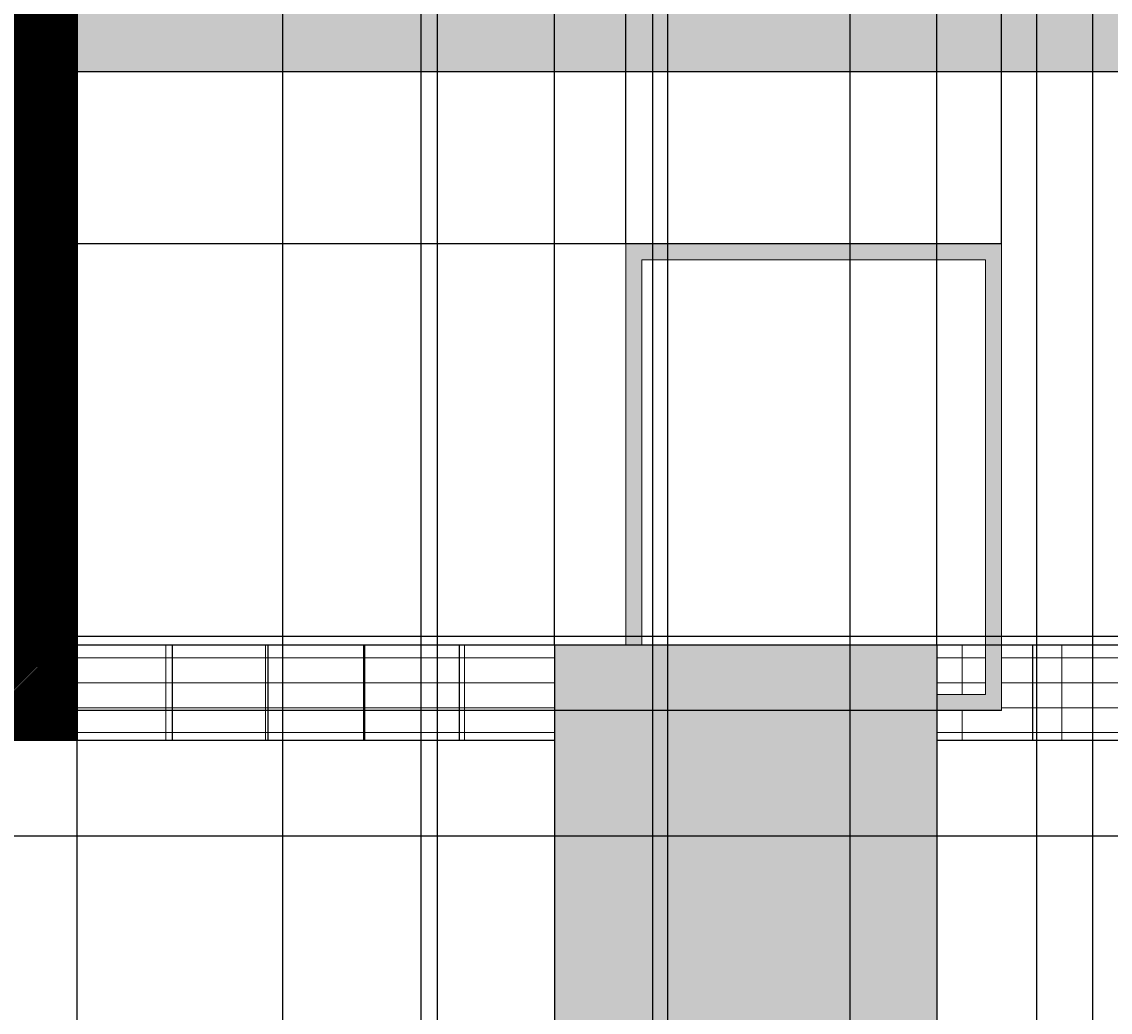
# Model space of a CAD drawing. Units: inches. Extents: x 484 to 1264, y 95 to 991.
# Tile 4 of 8: x 657 to 794, y 374 to 499. Entities that reach past the tile are written whole.
import ezdxf

# ---------------------------------------------------------------- set-up
doc = ezdxf.new("R2010")
doc.units = ezdxf.units.IN
doc.header["$MEASUREMENT"] = 0
for name, color, linetype, lineweight in [('A-ANNO-DIMS', 2, 'Continuous', 18), ('A-ELEV-TRIM', 7, 'Continuous', 18), ('A-GLAZ', 7, 'Continuous', 18), ('A-WALL', 7, 'Continuous', 35), ('L-FENC', 7, 'Continuous', 25), ('L-FENC-GRIL-PATT', 6, 'Continuous', 13)]:
    doc.layers.add(name, color=color, linetype=linetype, lineweight=lineweight)
for name, color, linetype, lineweight, true_color in [('A-ELEV-TRIM-PATT', 40, 'Continuous', 13, 0xe7c208), ('A-WALL-FRAM-PATT', 158, 'Continuous', 13, 0x131d3e), ('L-FENC-PATT', 34, 'Continuous', 13, 0xa25420)]:
    doc.layers.add(name, color=color, linetype=linetype, lineweight=lineweight, true_color=true_color)
doc.styles.get("Standard").update_dxf_attribs({"font": 'arial.ttf'})
doc.dimstyles.get("Standard").update_dxf_attribs({"dimtxt": 0.18, "dimasz": 0.18, "dimexe": 0.18, "dimexo": 0.0625, "dimgap": 0.09, "dimtad": 0, "dimtih": 1, "dimtoh": 1, "dimdec": 4, "dimzin": 0, "dimdsep": 46, "dimtxsty": 'Standard', "dimcen": 0.09, "dimadec": 0, "dimazin": 0, "dimtfac": 1, "dimtdec": 4, "dimtofl": 0, "dimtmove": 0, "dimatfit": 3, "dimfxl": 1, "dimtolj": 1, "dimtzin": 0, "dimarcsym": 0})

# ---------------------------------------------------------------- blocks, each defined once
blk = doc.blocks.new('*D16')
at = {"layer": 'A-ANNO-DIMS', "color": 0, "lineweight": -2, "transparency": 16777216}
for p, q in [((639.814711, 408.3220909999999), (639.814711, 94.79138999999998)), ((999.8147109999999, 318.322091), (999.8147109999999, 94.79138999999998)), ((639.9947109999999, 94.97139), (819.5262321459754, 94.97139)), ((999.634711, 94.97139), (820.1031898540245, 94.97139))]:
    blk.add_line(p, q, dxfattribs=at)
at = {"layer": 'A-ANNO-DIMS', "color": 0, "transparency": 16777216}
for points in [[(639.9947109999999, 95.00139), (639.9947109999999, 94.94139), (639.814711, 94.97139)], [(999.634711, 95.00139), (999.634711, 94.94139), (999.8147109999999, 94.97139)]]:
    blk.add_solid(points, dxfattribs=at)
at = {"layer": 'Defpoints', "color": 0, "transparency": 16777216}
for p in [(639.814711, 408.3845909999999), (999.8147109999999, 318.384591), (999.8147109999999, 94.97139)]:
    blk.add_point(p, dxfattribs=at)
at = {"layer": 'A-ANNO-DIMS', "color": 0, "transparency": 16777216, "insert": (819.814711, 94.97139), "char_height": 0.18, "attachment_point": 5}
blk.add_mtext('\\A1;360', dxfattribs=at)
blk = doc.blocks.new('*D17')
at = {"layer": 'A-ANNO-DIMS', "color": 0, "lineweight": -2, "transparency": 16777216}
for p, q in [((709.0057910000003, 950.0790140000004), (484.1461180000003, 950.0790140000004)), ((484.3261180000003, 949.8990140000005), (484.3261180000005, 628.4137670293318)), ((484.3261180000005, 306.5645910000001), (484.3261180000005, 628.0498379706688)), ((595.2596180000003, 306.3845910000001), (484.1461180000004, 306.3845910000001))]:
    blk.add_line(p, q, dxfattribs=at)
at = {"layer": 'A-ANNO-DIMS', "color": 0, "transparency": 16777216}
for points in [[(484.2961180000004, 949.8990140000005), (484.3561180000003, 949.8990140000005), (484.3261180000003, 950.0790140000004)], [(484.2961180000005, 306.5645910000001), (484.3561180000005, 306.5645910000001), (484.3261180000005, 306.3845910000001)]]:
    blk.add_solid(points, dxfattribs=at)
at = {"layer": 'Defpoints', "color": 0, "transparency": 16777216}
for p in [(484.3261180000003, 950.0790140000004), (709.0682910000002, 950.0790140000004), (595.3221180000002, 306.3845910000001)]:
    blk.add_point(p, dxfattribs=at)
at = {"layer": 'A-ANNO-DIMS', "color": 0, "transparency": 16777216, "insert": (484.3261180000005, 628.2318025000001), "char_height": 0.18, "attachment_point": 5}
blk.add_mtext('\\A1;643.7', dxfattribs=at)
blk = doc.blocks.new('*D18')
at = {"layer": 'A-ANNO-DIMS', "color": 0, "lineweight": -2, "transparency": 16777216}
for p, q in [((999.8772110000004, 501.3845910000002), (1264.083232000001, 501.3845910000003)), ((1263.903232000001, 501.2045910000002), (1263.903232000001, 404.0664941377902)), ((1263.903232000001, 306.5645910000002), (1263.903232000001, 403.7026878622103)), ((595.3846180000002, 306.3845910000001), (1264.083232000001, 306.3845910000002))]:
    blk.add_line(p, q, dxfattribs=at)
at = {"layer": 'A-ANNO-DIMS', "color": 0, "transparency": 16777216}
for points in [[(1263.873232000001, 501.2045910000002), (1263.933232000001, 501.2045910000002), (1263.903232000001, 501.3845910000003)], [(1263.873232000001, 306.5645910000002), (1263.933232000001, 306.5645910000002), (1263.903232000001, 306.3845910000002)]]:
    blk.add_solid(points, dxfattribs=at)
at = {"layer": 'Defpoints', "color": 0, "transparency": 16777216}
for p in [(999.8147110000004, 501.3845910000002), (1263.903232000001, 501.3845910000003), (595.3221180000002, 306.3845910000001)]:
    blk.add_point(p, dxfattribs=at)
at = {"layer": 'A-ANNO-DIMS', "color": 0, "transparency": 16777216, "insert": (1263.903232, 403.8845909999998), "char_height": 0.18, "attachment_point": 5}
blk.add_mtext('\\A1;195', dxfattribs=at)
blk = doc.blocks.new('*D23')
at = {"layer": 'A-ANNO-DIMS', "color": 0, "lineweight": -2, "transparency": 16777216}
for p, q in [((663.814711, 906.322091), (663.814711, 94.79139000000008)), ((709.068291, 889.0562129999998), (709.068291, 94.79139000000008)), ((663.9947109999999, 94.97139), (686.0434996357435, 94.97139)), ((708.8882910000001, 94.97139), (686.8395023642565, 94.97139))]:
    blk.add_line(p, q, dxfattribs=at)
at = {"layer": 'A-ANNO-DIMS', "color": 0, "transparency": 16777216}
for points in [[(663.9947109999999, 95.00139), (663.9947109999999, 94.94139), (663.814711, 94.97139)], [(708.8882910000001, 95.00139), (708.8882910000001, 94.94139), (709.068291, 94.97139)]]:
    blk.add_solid(points, dxfattribs=at)
at = {"layer": 'Defpoints', "color": 0, "transparency": 16777216}
for p in [(663.814711, 906.3845909999999), (709.068291, 889.118713), (709.068291, 94.97139)]:
    blk.add_point(p, dxfattribs=at)
at = {"layer": 'A-ANNO-DIMS', "color": 0, "transparency": 16777216, "insert": (686.441501, 94.97139), "char_height": 0.18, "attachment_point": 5}
blk.add_mtext('\\A1;45.25', dxfattribs=at)
blk = doc.blocks.new('*D24')
at = {"layer": 'A-ANNO-DIMS', "color": 0, "lineweight": -2, "transparency": 16777216}
for p, q in [((709.068291, 889.0562129999998), (709.068291, 94.79139000000008)), ((736.1200049999999, 889.0562129999998), (736.1200049999999, 94.79139000000008)), ((709.248291, 94.97139), (722.1982339481582, 94.97139)), ((735.940005, 94.97139), (722.9900620518417, 94.97139))]:
    blk.add_line(p, q, dxfattribs=at)
at = {"layer": 'A-ANNO-DIMS', "color": 0, "transparency": 16777216}
for points in [[(709.248291, 95.00139), (709.248291, 94.94139), (709.068291, 94.97139)], [(735.940005, 95.00139), (735.940005, 94.94139), (736.1200049999999, 94.97139)]]:
    blk.add_solid(points, dxfattribs=at)
at = {"layer": 'Defpoints', "color": 0, "transparency": 16777216}
for p in [(709.068291, 889.118713), (736.1200049999999, 889.118713), (736.1200049999999, 94.97139)]:
    blk.add_point(p, dxfattribs=at)
at = {"layer": 'A-ANNO-DIMS', "color": 0, "transparency": 16777216, "insert": (722.594148, 94.97139), "char_height": 0.18, "attachment_point": 5}
blk.add_mtext('\\A1;27.05', dxfattribs=at)
blk = doc.blocks.new('*D25')
at = {"layer": 'A-ANNO-DIMS', "color": 0, "lineweight": -2, "transparency": 16777216}
for p, q in [((736.1200049999999, 889.0562129999998), (736.1200049999999, 94.79139000000008)), ((760.86945, 889.0562129999998), (760.86945, 94.79139000000008)), ((736.3000049999999, 94.97139), (748.0988134481582, 94.97139)), ((760.6894500000001, 94.97139), (748.8906415518417, 94.97139))]:
    blk.add_line(p, q, dxfattribs=at)
at = {"layer": 'A-ANNO-DIMS', "color": 0, "transparency": 16777216}
for points in [[(736.3000049999999, 95.00139), (736.3000049999999, 94.94139), (736.1200049999999, 94.97139)], [(760.6894500000001, 95.00139), (760.6894500000001, 94.94139), (760.86945, 94.97139)]]:
    blk.add_solid(points, dxfattribs=at)
at = {"layer": 'Defpoints', "color": 0, "transparency": 16777216}
for p in [(736.1200049999999, 889.118713), (760.86945, 889.118713), (760.86945, 94.97139)]:
    blk.add_point(p, dxfattribs=at)
at = {"layer": 'A-ANNO-DIMS', "color": 0, "transparency": 16777216, "insert": (748.4947275, 94.97139), "char_height": 0.18, "attachment_point": 5}
blk.add_mtext('\\A1;24.75', dxfattribs=at)
blk = doc.blocks.new('*D26')
at = {"layer": 'A-ANNO-DIMS', "color": 0, "lineweight": -2, "transparency": 16777216}
for p, q in [((689.660436, 819.993689), (689.660436, 94.79139000000008)), ((663.814711, 810.322091), (663.814711, 94.79139000000008)), ((663.9947109999999, 94.97139), (676.2724711807639, 94.97139)), ((689.480436, 94.97139), (677.202675819236, 94.97139))]:
    blk.add_line(p, q, dxfattribs=at)
at = {"layer": 'A-ANNO-DIMS', "color": 0, "transparency": 16777216}
for points in [[(663.9947109999999, 95.00139), (663.9947109999999, 94.94139), (663.814711, 94.97139)], [(689.480436, 95.00139), (689.480436, 94.94139), (689.660436, 94.97139)]]:
    blk.add_solid(points, dxfattribs=at)
at = {"layer": 'Defpoints', "color": 0, "transparency": 16777216}
for p in [(689.660436, 820.0561889999999), (663.814711, 810.384591), (689.660436, 94.97139)]:
    blk.add_point(p, dxfattribs=at)
at = {"layer": 'A-ANNO-DIMS', "color": 0, "transparency": 16777216, "insert": (676.7375735, 94.97139), "char_height": 0.18, "attachment_point": 5}
blk.add_mtext('\\A1;25.846', dxfattribs=at)
blk = doc.blocks.new('*D27')
at = {"layer": 'A-ANNO-DIMS', "color": 0, "lineweight": -2, "transparency": 16777216}
for p, q in [((689.660436, 819.993689), (689.660436, 94.79139000000008)), ((737.977667, 819.993689), (737.977667, 94.79139000000008)), ((689.840436, 94.97139), (713.4226463158254, 94.97139)), ((737.797667, 94.97139), (714.2154566841745, 94.97139))]:
    blk.add_line(p, q, dxfattribs=at)
at = {"layer": 'A-ANNO-DIMS', "color": 0, "transparency": 16777216}
for points in [[(689.840436, 95.00139), (689.840436, 94.94139), (689.660436, 94.97139)], [(737.797667, 95.00139), (737.797667, 94.94139), (737.977667, 94.97139)]]:
    blk.add_solid(points, dxfattribs=at)
at = {"layer": 'Defpoints', "color": 0, "transparency": 16777216}
for p in [(689.660436, 820.0561889999999), (737.977667, 820.0561889999999), (737.977667, 94.97139)]:
    blk.add_point(p, dxfattribs=at)
at = {"layer": 'A-ANNO-DIMS', "color": 0, "transparency": 16777216, "insert": (713.8190514999999, 94.97139), "char_height": 0.18, "attachment_point": 5}
blk.add_mtext('\\A1;48.32', dxfattribs=at)
blk = doc.blocks.new('*D28')
at = {"layer": 'A-ANNO-DIMS', "color": 0, "lineweight": -2, "transparency": 16777216}
for p, q in [((737.977667, 819.993689), (737.977667, 94.79139000000008)), ((784.302445, 819.993689), (784.302445, 94.79139000000008)), ((738.157667, 94.97139), (760.6721296698499, 94.97139)), ((784.1224450000001, 94.97139), (761.6079823301499, 94.97139))]:
    blk.add_line(p, q, dxfattribs=at)
at = {"layer": 'A-ANNO-DIMS', "color": 0, "transparency": 16777216}
for points in [[(738.157667, 95.00139), (738.157667, 94.94139), (737.977667, 94.97139)], [(784.1224450000001, 95.00139), (784.1224450000001, 94.94139), (784.302445, 94.97139)]]:
    blk.add_solid(points, dxfattribs=at)
at = {"layer": 'Defpoints', "color": 0, "transparency": 16777216}
for p in [(737.977667, 820.0561889999999), (784.302445, 820.0561889999999), (784.302445, 94.97139)]:
    blk.add_point(p, dxfattribs=at)
at = {"layer": 'A-ANNO-DIMS', "color": 0, "transparency": 16777216, "insert": (761.1400559999998, 94.97139), "char_height": 0.18, "attachment_point": 5}
blk.add_mtext('\\A1;46.325', dxfattribs=at)
blk = doc.blocks.new('*D29')
at = {"layer": 'A-ANNO-DIMS', "color": 0, "lineweight": -2, "transparency": 16777216}
for p, q in [((831.8147109999999, 906.322091), (831.8147109999999, 94.79139000000008)), ((784.302445, 819.993689), (784.302445, 94.79139000000008)), ((784.4824449999999, 94.97139), (807.6786257489769, 94.97139)), ((831.634711, 94.97139), (808.438530251023, 94.97139))]:
    blk.add_line(p, q, dxfattribs=at)
at = {"layer": 'A-ANNO-DIMS', "color": 0, "transparency": 16777216}
for points in [[(784.4824449999999, 95.00139), (784.4824449999999, 94.94139), (784.302445, 94.97139)], [(831.634711, 95.00139), (831.634711, 94.94139), (831.8147109999999, 94.97139)]]:
    blk.add_solid(points, dxfattribs=at)
at = {"layer": 'Defpoints', "color": 0, "transparency": 16777216}
for p in [(831.8147109999999, 906.3845909999999), (784.302445, 820.0561889999999), (831.8147109999999, 94.97139)]:
    blk.add_point(p, dxfattribs=at)
at = {"layer": 'A-ANNO-DIMS', "color": 0, "transparency": 16777216, "insert": (808.0585779999999, 94.97139), "char_height": 0.18, "attachment_point": 5}
blk.add_mtext('\\A1;47.51', dxfattribs=at)
blk = doc.blocks.new('*D33')
at = {"layer": 'A-ANNO-DIMS', "color": 0, "lineweight": -2, "transparency": 16777216}
for p, q in [((639.814711, 930.322091), (639.814711, 94.79139000000008)), ((663.814711, 810.322091), (663.814711, 94.79139000000008)), ((639.9947109999999, 94.97139), (651.5946223233287, 94.97139)), ((663.634711, 94.97139), (652.0347996766712, 94.97139))]:
    blk.add_line(p, q, dxfattribs=at)
at = {"layer": 'A-ANNO-DIMS', "color": 0, "transparency": 16777216}
for points in [[(639.9947109999999, 95.00139), (639.9947109999999, 94.94139), (639.814711, 94.97139)], [(663.634711, 95.00139), (663.634711, 94.94139), (663.814711, 94.97139)]]:
    blk.add_solid(points, dxfattribs=at)
at = {"layer": 'Defpoints', "color": 0, "transparency": 16777216}
for p in [(639.814711, 930.3845909999999), (663.814711, 810.384591), (663.814711, 94.97139)]:
    blk.add_point(p, dxfattribs=at)
at = {"layer": 'A-ANNO-DIMS', "color": 0, "transparency": 16777216, "insert": (651.814711, 94.97139), "char_height": 0.18, "attachment_point": 5}
blk.add_mtext('\\A1;24', dxfattribs=at)
blk = doc.blocks.new('*D36')
at = {"layer": 'A-ANNO-DIMS', "color": 0, "lineweight": -2, "transparency": 16777216}
for p, q in [((707.0379609999999, 581.213901), (707.0379609999999, 94.79138999999998)), ((663.814711, 501.322091), (663.814711, 94.79138999999998)), ((663.9947109999999, 94.97139), (685.0299308158254, 94.97139)), ((706.857961, 94.97139), (685.8227411841744, 94.97139))]:
    blk.add_line(p, q, dxfattribs=at)
at = {"layer": 'A-ANNO-DIMS', "color": 0, "transparency": 16777216}
for points in [[(663.9947109999999, 95.00139), (663.9947109999999, 94.94139), (663.814711, 94.97139)], [(706.857961, 95.00139), (706.857961, 94.94139), (707.0379609999999, 94.97139)]]:
    blk.add_solid(points, dxfattribs=at)
at = {"layer": 'Defpoints', "color": 0, "transparency": 16777216}
for p in [(707.0379609999999, 581.2764009999999), (663.814711, 501.3845909999999), (707.0379609999999, 94.97139)]:
    blk.add_point(p, dxfattribs=at)
at = {"layer": 'A-ANNO-DIMS', "color": 0, "transparency": 16777216, "insert": (685.426336, 94.97139), "char_height": 0.18, "attachment_point": 5}
blk.add_mtext('\\A1;43.22', dxfattribs=at)
blk = doc.blocks.new('*D37')
at = {"layer": 'A-ANNO-DIMS', "color": 0, "lineweight": -2, "transparency": 16777216}
for p, q in [((707.0379609999999, 581.213901), (707.0379609999999, 94.79138999999998)), ((791.360463, 581.213901), (791.360463, 94.79138999999998)), ((707.217961, 94.97139), (748.8063061336971, 94.97139)), ((791.180463, 94.97139), (749.5921178663028, 94.97139))]:
    blk.add_line(p, q, dxfattribs=at)
at = {"layer": 'A-ANNO-DIMS', "color": 0, "transparency": 16777216}
for points in [[(707.217961, 95.00139), (707.217961, 94.94139), (707.0379609999999, 94.97139)], [(791.180463, 95.00139), (791.180463, 94.94139), (791.360463, 94.97139)]]:
    blk.add_solid(points, dxfattribs=at)
at = {"layer": 'Defpoints', "color": 0, "transparency": 16777216}
for p in [(707.0379609999999, 581.2764009999999), (791.360463, 581.2764009999999), (791.360463, 94.97139)]:
    blk.add_point(p, dxfattribs=at)
at = {"layer": 'A-ANNO-DIMS', "color": 0, "transparency": 16777216, "insert": (749.1992119999999, 94.97139), "char_height": 0.18, "attachment_point": 5}
blk.add_mtext('\\A1;84.32', dxfattribs=at)
blk = doc.blocks.new('*D45')
at = {"layer": 'A-ANNO-DIMS', "color": 0, "lineweight": -2, "transparency": 16777216}
for p, q in [((732.774432, 470.825236), (732.774432, 991.109014)), ((732.954432, 990.929014), (755.9435934427012, 990.929014)), ((779.7274070000001, 990.929014), (756.7382455572988, 990.929014)), ((779.907407, 470.825236), (779.907407, 991.109014))]:
    blk.add_line(p, q, dxfattribs=at)
at = {"layer": 'A-ANNO-DIMS', "color": 0, "transparency": 16777216}
for points in [[(732.954432, 990.959014), (732.954432, 990.899014), (732.774432, 990.929014)], [(779.7274070000001, 990.959014), (779.7274070000001, 990.899014), (779.907407, 990.929014)]]:
    blk.add_solid(points, dxfattribs=at)
at = {"layer": 'Defpoints', "color": 0, "transparency": 16777216}
for p in [(779.907407, 990.929014), (732.774432, 470.762736), (779.907407, 470.762736)]:
    blk.add_point(p, dxfattribs=at)
at = {"layer": 'A-ANNO-DIMS', "color": 0, "transparency": 16777216, "insert": (756.3409195, 990.929014), "char_height": 0.18, "attachment_point": 5}
blk.add_mtext('\\A1;47.13', dxfattribs=at)
blk = doc.blocks.new('*D46')
at = {"layer": 'A-ANNO-DIMS', "color": 0, "lineweight": -2, "transparency": 16777216}
for p, q in [((779.907407, 470.825236), (779.907407, 991.109014)), ((780.0874069999999, 990.929014), (805.4847288499319, 990.929014)), ((831.634711, 990.929014), (806.2373891500682, 990.929014)), ((831.8147109999999, 492.447091), (831.8147109999999, 991.109014))]:
    blk.add_line(p, q, dxfattribs=at)
at = {"layer": 'A-ANNO-DIMS', "color": 0, "transparency": 16777216}
for points in [[(780.0874069999999, 990.959014), (780.0874069999999, 990.899014), (779.907407, 990.929014)], [(831.634711, 990.959014), (831.634711, 990.899014), (831.8147109999999, 990.929014)]]:
    blk.add_solid(points, dxfattribs=at)
at = {"layer": 'Defpoints', "color": 0, "transparency": 16777216}
for p in [(831.8147109999999, 990.929014), (831.8147109999999, 492.3845909999999), (779.907407, 470.762736)]:
    blk.add_point(p, dxfattribs=at)
at = {"layer": 'A-ANNO-DIMS', "color": 0, "transparency": 16777216, "insert": (805.861059, 990.929014), "char_height": 0.18, "attachment_point": 5}
blk.add_mtext('\\A1;51.91', dxfattribs=at)
blk = doc.blocks.new('*D47')
at = {"layer": 'A-ANNO-DIMS', "color": 0, "lineweight": -2, "transparency": 16777216}
for p, q in [((779.8449070000004, 470.7627360000002), (484.1461180000004, 470.7627360000001)), ((484.3261180000005, 470.5827360000001), (484.3261180000005, 441.64267863779)), ((484.3261180000005, 412.3388150000002), (484.3261180000005, 441.2788723622102)), ((779.8449070000004, 412.1588150000002), (484.1461180000004, 412.1588150000001))]:
    blk.add_line(p, q, dxfattribs=at)
at = {"layer": 'A-ANNO-DIMS', "color": 0, "transparency": 16777216}
for points in [[(484.2961180000004, 470.5827360000001), (484.3561180000004, 470.5827360000001), (484.3261180000005, 470.7627360000001)], [(484.2961180000004, 412.3388150000002), (484.3561180000004, 412.3388150000002), (484.3261180000005, 412.1588150000001)]]:
    blk.add_solid(points, dxfattribs=at)
at = {"layer": 'Defpoints', "color": 0, "transparency": 16777216}
for p in [(484.3261180000005, 470.7627360000001), (779.9074070000004, 470.7627360000002), (779.9074070000004, 412.1588150000002)]:
    blk.add_point(p, dxfattribs=at)
at = {"layer": 'A-ANNO-DIMS', "color": 0, "transparency": 16777216, "insert": (484.3261180000005, 441.4607754999998), "char_height": 0.18, "attachment_point": 5}
blk.add_mtext('\\A1;58.6', dxfattribs=at)
blk = doc.blocks.new('*D48')
at = {"layer": 'A-ANNO-DIMS', "color": 0, "lineweight": -2, "transparency": 16777216}
for p, q in [((831.7522110000004, 492.3845910000002), (484.1461180000004, 492.3845910000001)), ((484.3261180000005, 492.2045910000001), (484.3261180000005, 481.75556663779)), ((484.3261180000005, 470.9427360000002), (484.3261180000005, 481.3917603622102)), ((779.8449070000004, 470.7627360000002), (484.1461180000004, 470.7627360000001))]:
    blk.add_line(p, q, dxfattribs=at)
at = {"layer": 'A-ANNO-DIMS', "color": 0, "transparency": 16777216}
for points in [[(484.2961180000004, 492.2045910000001), (484.3561180000004, 492.2045910000001), (484.3261180000005, 492.3845910000001)], [(484.2961180000004, 470.9427360000002), (484.3561180000004, 470.9427360000002), (484.3261180000005, 470.7627360000001)]]:
    blk.add_solid(points, dxfattribs=at)
at = {"layer": 'Defpoints', "color": 0, "transparency": 16777216}
for p in [(484.3261180000005, 492.3845910000001), (831.8147110000004, 492.3845910000002), (779.9074070000004, 470.7627360000002)]:
    blk.add_point(p, dxfattribs=at)
at = {"layer": 'A-ANNO-DIMS', "color": 0, "transparency": 16777216, "insert": (484.3261180000005, 481.5736634999999), "char_height": 0.18, "attachment_point": 5}
blk.add_mtext('\\A1;21.62', dxfattribs=at)
blk = doc.blocks.new('*D51')
at = {"layer": 'A-ANNO-DIMS', "color": 0, "lineweight": -2, "transparency": 16777216}
for p, q in [((869.5523070000005, 421.4725140000002), (484.1461180000004, 421.4725140000001)), ((484.3261180000004, 421.2925140000001), (484.3261180000005, 370.1105170293316)), ((484.3261180000005, 318.5645910000001), (484.3261180000005, 369.7465879706685)), ((855.7522110000004, 318.3845910000001), (484.1461180000004, 318.384591))]:
    blk.add_line(p, q, dxfattribs=at)
at = {"layer": 'A-ANNO-DIMS', "color": 0, "transparency": 16777216}
for points in [[(484.2961180000004, 421.2925140000001), (484.3561180000003, 421.2925140000001), (484.3261180000004, 421.4725140000001)], [(484.2961180000004, 318.5645910000001), (484.3561180000004, 318.5645910000001), (484.3261180000005, 318.384591)]]:
    blk.add_solid(points, dxfattribs=at)
at = {"layer": 'Defpoints', "color": 0, "transparency": 16777216}
for p in [(484.3261180000004, 421.4725140000001), (869.6148070000004, 421.4725140000002), (855.8147110000004, 318.3845910000001)]:
    blk.add_point(p, dxfattribs=at)
at = {"layer": 'A-ANNO-DIMS', "color": 0, "transparency": 16777216, "insert": (484.3261180000004, 369.9285524999999), "char_height": 0.18, "attachment_point": 5}
blk.add_mtext('\\A1;103.09', dxfattribs=at)
blk = doc.blocks.new('*D52')
at = {"layer": 'A-ANNO-DIMS', "color": 0, "lineweight": -2, "transparency": 16777216}
for p, q in [((723.8147109999999, 420.447091), (723.8147109999999, 991.109014)), ((723.9947109999999, 990.929014), (747.5919824870394, 990.929014)), ((771.634711, 990.929014), (748.0374395129604, 990.929014)), ((771.814711, 420.447091), (771.814711, 991.109014))]:
    blk.add_line(p, q, dxfattribs=at)
at = {"layer": 'A-ANNO-DIMS', "color": 0, "transparency": 16777216}
for points in [[(723.9947109999999, 990.959014), (723.9947109999999, 990.899014), (723.8147109999999, 990.929014)], [(771.634711, 990.959014), (771.634711, 990.899014), (771.814711, 990.929014)]]:
    blk.add_solid(points, dxfattribs=at)
at = {"layer": 'Defpoints', "color": 0, "transparency": 16777216}
for p in [(771.814711, 990.929014), (723.8147109999999, 420.384591), (771.814711, 420.384591)]:
    blk.add_point(p, dxfattribs=at)
at = {"layer": 'A-ANNO-DIMS', "color": 0, "transparency": 16777216, "insert": (747.814711, 990.929014), "char_height": 0.18, "attachment_point": 5}
blk.add_mtext('\\A1;48', dxfattribs=at)
blk = doc.blocks.new('*D58')
at = {"layer": 'A-ANNO-DIMS', "color": 0, "lineweight": -2, "transparency": 16777216}
for p, q in [((855.7522110000004, 396.3845910000003), (484.1461180000004, 396.3845910000001)), ((484.3261180000004, 396.2045910000002), (484.3261180000005, 363.56649413779)), ((484.3261180000005, 330.5645910000001), (484.3261180000005, 363.2026878622101)), ((855.7522110000004, 330.3845910000001), (484.1461180000004, 330.3845910000001))]:
    blk.add_line(p, q, dxfattribs=at)
at = {"layer": 'A-ANNO-DIMS', "color": 0, "transparency": 16777216}
for points in [[(484.2961180000004, 396.2045910000002), (484.3561180000003, 396.2045910000002), (484.3261180000004, 396.3845910000001)], [(484.2961180000004, 330.5645910000001), (484.3561180000004, 330.5645910000001), (484.3261180000005, 330.3845910000001)]]:
    blk.add_solid(points, dxfattribs=at)
at = {"layer": 'Defpoints', "color": 0, "transparency": 16777216}
for p in [(484.3261180000004, 396.3845910000001), (855.8147110000004, 396.3845910000003), (855.8147110000004, 330.3845910000001)]:
    blk.add_point(p, dxfattribs=at)
at = {"layer": 'A-ANNO-DIMS', "color": 0, "transparency": 16777216, "insert": (484.3261180000004, 363.3845909999998), "char_height": 0.18, "attachment_point": 5}
blk.add_mtext('\\A1;66', dxfattribs=at)

msp = doc.modelspace()

# ---------------------------------------------------------------- hatches: boundary and pattern name
at = {"layer": 'A-ELEV-TRIM-PATT'}
h = msp.add_hatch(color=256, dxfattribs=at)
h.dxf.hatch_style = 1
h.paths.add_polyline_path([(791.3604632189817, 737.6508125955456), (707.0379608801577, 737.6508125955456), (707.0379608801577, 581.2764007961791), (791.3604632189817, 581.2764007961791)])
h.paths.add_polyline_path([(789.3604632189817, 735.6508125955456), (789.3604632189817, 583.2764007961791), (709.0379608801576, 583.2764007961791), (709.0379608801576, 735.6508125955456)], flags=16)
h.paths.add_polyline_path([(850.1751791371953, 699.3334200613348), (840.6400557475826, 699.3334200613348), (840.6400557475826, 681.6081848608055), (850.1751791371953, 681.6081848608055)])
h.paths.add_polyline_path([(850.9809155201601, 648.8446729214583), (839.9452998180949, 648.8446729214583), (839.9452998180949, 628.2142842352996), (850.9809155201601, 628.2142842352996)])
h.paths.add_polyline_path([(849.2080120719693, 595.8058680326312), (838.5283820280656, 595.8058680326312), (838.5283820280656, 577.665356669208), (849.2080120719693, 577.665356669208)])
h.paths.add_polyline_path([(723.4575003799, 950.0790139985864), (709.0682911431468, 950.0790139985864), (709.0682911431468, 889.1187126845098), (723.4575003799, 889.1187126845098)])
h.paths.add_polyline_path([(750.5092145489798, 950.0790139985864), (736.1200053122265, 950.0790139985864), (736.1200053122265, 889.1187126845098), (750.5092145489798, 889.1187126845098)])
h.paths.add_polyline_path([(775.2586596621131, 950.0790139985864), (760.8694504253598, 950.0790139985864), (760.8694504253598, 889.1187126845098), (775.2586596621131, 889.1187126845098)])
h.paths.add_polyline_path([(759.8947585294499, 859.8728276012089), (737.9776673698088, 859.8728276012089), (737.9776673698088, 820.0561886043143), (759.8947585294499, 820.0561886043143)])
h.paths.add_polyline_path([(757.89475852945, 822.0561886043142), (739.9776673698088, 822.0561886043142), (739.9776673698088, 857.8728276012089), (757.89475852945, 857.8728276012089)], flags=16)
h.paths.add_polyline_path([(806.2195360287933, 859.8728276012089), (784.302444869152, 859.8728276012089), (784.302444869152, 820.0561886043143), (806.2195360287933, 820.0561886043143)])
h.paths.add_polyline_path([(786.302444869152, 857.8728276012089), (804.2195360287932, 857.8728276012089), (804.2195360287932, 822.0561886043142), (786.302444869152, 822.0561886043142)], flags=16)
h.paths.add_polyline_path([(711.5775266940199, 859.8728276012089), (689.6604355343788, 859.8728276012089), (689.6604355343788, 820.0561886043143), (711.5775266940199, 820.0561886043143)])
h.paths.add_polyline_path([(709.57752669402, 822.0561886043142), (691.6604355343788, 822.0561886043142), (691.6604355343788, 857.8728276012089), (709.57752669402, 857.8728276012089)], flags=16)
h.paths.add_polyline_path([(831.8147106526719, 810.3845910111976), (663.814710652672, 810.3845910111976), (663.814710652672, 801.3845910111976), (831.8147106526719, 801.3845910111978)])
h.paths.add_polyline_path([(831.8147106526719, 501.3845910111976), (663.814710652672, 501.3845910111978), (663.814710652672, 492.3845910111977), (831.8147106526719, 492.3845910111977)])
h.paths.add_polyline_path([(779.9074070481965, 470.7627364727195), (732.7744315549462, 470.7627364727195), (732.7744315549462, 420.3845910111978), (734.7744315549462, 420.3845910111978), (734.7744315549462, 468.7627364727195), (777.9074070481965, 468.7627364727195), (777.9074070481965, 420.3845910111978), (779.9074070481965, 420.3845910111978)])
h.paths.add_polyline_path([(779.9074070481965, 420.3845910111978), (777.9074070481965, 420.3845910111978), (777.9074070481965, 414.1588149678183), (771.814710652672, 414.1588149678181), (771.814710652672, 412.1588149678181), (779.9074070481965, 412.1588149678181)])
at = {"layer": 'A-WALL-FRAM-PATT'}
h = msp.add_hatch(dxfattribs=at)
h.set_pattern_fill('ANSI31', color=256)
h.set_pattern_definition([(45, (0, 0), (-0.0883883476483185, 0.0883883476483185), [])])
h.paths.add_polyline_path([(999.8147106526721, 810.3845910111976), (831.8147106526719, 810.3845910111976), (831.8147106526719, 501.3845910111976), (999.8147106526721, 501.3845910111976), (999.8147106526721, 537.3845910111977), (855.8147106526718, 537.3845910111977), (855.8147106526719, 705.3845910111976), (999.8147106526721, 705.3845910111976)])
h.paths.add_polyline_path([(850.1751791371953, 699.3334200613348), (850.1751791371953, 681.6081848608055), (840.6400557475826, 681.6081848608055), (840.6400557475826, 699.3334200613348)], flags=16)
h.paths.add_polyline_path([(850.9809155201601, 648.8446729214583), (850.9809155201601, 628.2142842352996), (839.9452998180949, 628.2142842352996), (839.9452998180949, 648.8446729214583)], flags=16)
h.paths.add_polyline_path([(849.2080120719693, 595.8058680326312), (849.2080120719693, 577.665356669208), (838.5283820280656, 577.665356669208), (838.5283820280656, 595.8058680326312)], flags=16)
h.paths.add_polyline_path([(663.814710652672, 906.3845910111977), (709.0682911431468, 906.3845910111977), (709.0682911431468, 930.3845910111977), (639.8147106526721, 930.3845910111977), (639.814710652672, 408.3845910111977), (663.814710652672, 408.3845910111977)])
h.paths.add_polyline_path([(885.814710652672, 930.3845910111977), (775.2586596621131, 930.3845910111977), (775.2586596621131, 906.3845910111977), (885.814710652672, 906.3845910111977)])
h.paths.add_polyline_path([(760.8694504253598, 930.3845910111977), (750.5092145489798, 930.3845910111977), (750.5092145489798, 906.3845910111977), (760.8694504253598, 906.3845910111977)])
h.paths.add_polyline_path([(736.1200053122265, 930.3845910111977), (723.4575003799, 930.3845910111977), (723.4575003799, 906.3845910111977), (736.1200053122265, 906.3845910111977)])
at = {"layer": 'L-FENC-GRIL-PATT'}
h = msp.add_hatch(dxfattribs=at)
h.set_pattern_fill('GRATE', color=256, scale=100)
h.set_pattern_definition([(0, (0, 0), (0, 3.125), []), (90, (0, 0), (-12.5, 8e-16), [])])
h.paths.add_polyline_path([(974.8147106526721, 396.3845910111977), (927.8147106526721, 396.3845910111978), (927.814710652672, 330.3845910111977), (974.8147106526719, 330.3845910111978)])
h.paths.add_polyline_path([(903.8147106526721, 396.3845910111981), (855.8147106526719, 396.3845910111981), (855.8147106526719, 330.3845910111977), (903.814710652672, 330.3845910111976)])
h.paths.add_polyline_path([(819.814710652672, 420.3845910111978), (807.8147106526721, 420.3845910111978), (807.8147106526721, 408.3845910111977), (819.8147106526718, 408.3845910111977)])
h.paths.add_polyline_path([(807.8147106526721, 420.3845910111978), (795.814710652672, 420.3845910111978), (795.8147106526719, 408.3845910111978), (807.8147106526721, 408.3845910111977)])
h.paths.add_polyline_path([(795.814710652672, 420.3845910111978), (783.814710652672, 420.3845910111978), (783.8147106526719, 408.3845910111978), (795.8147106526719, 408.3845910111978)])
h.paths.add_polyline_path([(831.8147106526719, 420.3845910111978), (819.814710652672, 420.3845910111978), (819.8147106526718, 408.3845910111977), (831.8147106526719, 408.3845910111977)])
h.paths.add_polyline_path([(783.814710652672, 420.3845910111978), (779.9104622014929, 420.3845910111978), (779.9104622014929, 412.1379508589634), (771.814710652672, 412.1379508589634), (771.814710652672, 408.3845910111978), (783.8147106526719, 408.3845910111978)])
h.paths.add_polyline_path([(777.9104622014929, 420.3845910111978), (771.814710652672, 420.3845910111978), (771.814710652672, 414.1379508589634), (777.9104622014929, 414.1379508589634)], flags=17)
h.paths.add_polyline_path([(723.8147106526721, 420.3845910111978), (711.8147106526721, 420.3845910111978), (711.814710652672, 408.3845910111978), (723.8147106526721, 408.3845910111978)])
h.paths.add_polyline_path([(711.8147106526721, 420.3845910111978), (699.814710652672, 420.3845910111978), (699.814710652672, 408.3845910111978), (711.814710652672, 408.3845910111978)])
h.paths.add_polyline_path([(699.814710652672, 420.3845910111978), (687.814710652672, 420.3845910111978), (687.814710652672, 408.3845910111978), (699.814710652672, 408.3845910111978)])
h.paths.add_polyline_path([(687.814710652672, 420.3845910111978), (675.814710652672, 420.3845910111978), (675.814710652672, 408.3845910111978), (687.814710652672, 408.3845910111978)])
h.paths.add_polyline_path([(675.814710652672, 420.3845910111978), (663.8147106526719, 420.3845910111978), (663.814710652672, 408.3845910111977), (675.814710652672, 408.3845910111978)])
h.paths.add_polyline_path([(639.814710652672, 420.3845910111978), (631.3221178064251, 420.3845910111978), (631.3221178064249, 408.3845910111977), (639.814710652672, 408.3845910111977)])
h.paths.add_polyline_path([(631.3221178064251, 420.3845910111978), (619.3221178064249, 420.3845910111978), (619.3221178064249, 408.3845910111977), (631.3221178064249, 408.3845910111977)])
at = {"layer": 'L-FENC-PATT'}
h = msp.add_hatch(color=256, dxfattribs=at)
h.dxf.hatch_style = 1
h.paths.add_polyline_path([(619.3221178064251, 420.3845910111978), (595.3221178064251, 420.3845910111978), (595.3221178064248, 306.3845910111977), (855.8147106526719, 306.3845910111977), (855.8147106526719, 420.3845910111978), (831.8147106526719, 420.3845910111978), (831.8147106526719, 330.3845910111977), (771.8147106526721, 330.3845910111976), (771.814710652672, 420.3845910111978), (723.8147106526721, 420.3845910111978), (723.814710652672, 330.3845910111976), (619.3221178064249, 330.3845910111977)])
h.paths.add_polyline_path([(999.8147106526721, 420.3845910111977), (975.814710652672, 420.3845910111978), (975.8147106526719, 318.3845910111977), (999.8147106526719, 318.3845910111977)])

# ---------------------------------------------------------------- linework, layer by layer
at = {"layer": 'A-ELEV-TRIM'}
msp.add_line((831.8147106526719, 492.3845910111977), (663.814710652672, 492.3845910111977), dxfattribs=at)
at = {"layer": 'A-GLAZ'}
for points in [[(732.7744315549462, 420.3845910111978), (732.7744315549462, 470.7627364727195), (779.9074070481965, 470.7627364727195), (779.9074070481965, 412.1588149678181), (771.814710652672, 412.1588149678181)], [(734.7744315549462, 420.3845910111978), (734.7744315549462, 468.7627364727195), (777.9074070481965, 468.7627364727195), (777.9074070481965, 414.1588149678182), (771.814710652672, 414.1588149678182)]]:
    msp.add_lwpolyline(points, dxfattribs=at)
at = {"layer": 'A-WALL'}
msp.add_line((663.814710652672, 906.3845910111977), (663.814710652672, 408.3845910111977), dxfattribs=at)
at = {"layer": 'L-FENC'}
for p, q in [((855.8147106526719, 420.3845910111978), (663.814710652672, 420.3845910111978)), ((675.814710652672, 420.3845910111978), (675.814710652672, 408.3845910111977)), ((687.814710652672, 420.3845910111978), (687.814710652672, 408.3845910111977)), ((699.814710652672, 420.3845910111978), (699.814710652672, 408.3845910111977)), ((711.8147106526721, 420.3845910111978), (711.814710652672, 408.3845910111977)), ((723.8147106526721, 420.3845910111978), (723.814710652672, 330.3845910111976)), ((771.814710652672, 420.3845910111978), (771.8147106526721, 330.3845910111976)), ((783.814710652672, 420.3845910111978), (783.8147106526719, 408.3845910111978)), ((723.8147106526721, 408.3845910111978), (619.3221178064252, 408.3845910111977)), ((831.8147106526719, 408.3845910111977), (771.8147106526721, 408.3845910111978))]:
    msp.add_line(p, q, dxfattribs=at)

# ---------------------------------------------------------------- dimensions: what is measured, and where the dimension line sits
at = {"layer": 'A-ANNO-DIMS'}
for base, p1, p2, override, picture, middle in [((771.814711, 990.929014), (723.8147109999999, 420.384591), (771.814711, 420.384591), {"dimdec": 0, "dimlfac": 1, "dimrnd": 0, "dimzin": 0, "dimdsep": 46, "dimlunit": 2}, '*D52', (747.814711, 990.929014)), ((779.907407, 990.929014), (732.774432, 470.762736), (779.907407, 470.762736), {"dimdec": 2, "dimlfac": 1, "dimrnd": 0, "dimzin": 0, "dimdsep": 46, "dimlunit": 2}, '*D45', (756.3409195, 990.929014)), ((831.8147109999999, 990.929014), (779.907407, 470.762736), (831.8147109999999, 492.3845909999999), {"dimdec": 2, "dimlfac": 1, "dimrnd": 0, "dimzin": 0, "dimdsep": 46, "dimlunit": 2}, '*D46', (805.861059, 990.929014)), ((663.814711, 94.97139), (639.814711, 930.3845909999999), (663.814711, 810.384591), {"dimdec": 0, "dimlfac": 1, "dimrnd": 0, "dimzin": 0, "dimdsep": 46, "dimlunit": 2}, '*D33', (651.814711, 94.97139)), ((709.068291, 94.97139), (663.814711, 906.3845909999999), (709.068291, 889.118713), {"dimdec": 2, "dimlfac": 1, "dimrnd": 0, "dimzin": 0, "dimdsep": 46, "dimlunit": 2}, '*D23', (686.441501, 94.97139)), ((831.8147109999999, 94.97139), (784.302445, 820.0561889999999), (831.8147109999999, 906.3845909999999), {"dimdec": 2, "dimlfac": 1, "dimrnd": 0, "dimzin": 0, "dimdsep": 46, "dimlunit": 2}, '*D29', (808.0585779999999, 94.97139)), ((736.1200049999999, 94.97139), (709.068291, 889.118713), (736.1200049999999, 889.118713), {"dimdec": 2, "dimlfac": 1, "dimrnd": 0, "dimzin": 0, "dimdsep": 46, "dimlunit": 2}, '*D24', (722.594148, 94.97139)), ((760.86945, 94.97139), (736.1200049999999, 889.118713), (760.86945, 889.118713), {"dimdec": 2, "dimlfac": 1, "dimrnd": 0, "dimzin": 0, "dimdsep": 46, "dimlunit": 2}, '*D25', (748.4947275, 94.97139)), ((689.660436, 94.97139), (663.814711, 810.384591), (689.660436, 820.0561889999999), {"dimdec": 3, "dimlfac": 1, "dimrnd": 0, "dimzin": 0, "dimdsep": 46, "dimlunit": 2}, '*D26', (676.7375735, 94.97139)), ((737.977667, 94.97139), (689.660436, 820.0561889999999), (737.977667, 820.0561889999999), {"dimdec": 2, "dimlfac": 1, "dimrnd": 0, "dimzin": 0, "dimdsep": 46, "dimlunit": 2}, '*D27', (713.8190514999999, 94.97139)), ((784.302445, 94.97139), (737.977667, 820.0561889999999), (784.302445, 820.0561889999999), {"dimdec": 3, "dimlfac": 1, "dimrnd": 0, "dimzin": 0, "dimdsep": 46, "dimlunit": 2}, '*D28', (761.1400559999998, 94.97139)), ((707.0379609999999, 94.97139), (663.814711, 501.3845909999999), (707.0379609999999, 581.2764009999999), {"dimdec": 2, "dimlfac": 1, "dimrnd": 0, "dimzin": 0, "dimdsep": 46, "dimlunit": 2}, '*D36', (685.426336, 94.97139)), ((791.360463, 94.97139), (707.0379609999999, 581.2764009999999), (791.360463, 581.2764009999999), {"dimdec": 2, "dimlfac": 1, "dimrnd": 0, "dimzin": 0, "dimdsep": 46, "dimlunit": 2}, '*D37', (749.1992119999999, 94.97139)), ((999.8147109999999, 94.97139), (639.814711, 408.3845909999999), (999.8147109999999, 318.384591), {"dimdec": 0, "dimlfac": 1, "dimrnd": 0, "dimzin": 0, "dimdsep": 46, "dimlunit": 2}, '*D16', (819.814711, 94.97139))]:
    dim = msp.add_linear_dim(base=base, p1=p1, p2=p2, dimstyle='Standard', override=override, dxfattribs=at)
    dim.commit()
    dim.dimension.update_dxf_attribs({"geometry": picture, "text_midpoint": middle})
for base, p1, p2, override, picture, middle in [((484.3261180000003, 950.0790140000004), (595.322118, 306.384591), (709.068291, 950.0790140000001), {"dimdec": 1, "dimlfac": 1, "dimrnd": 0, "dimzin": 0, "dimdsep": 46, "dimlunit": 2}, '*D17', (484.3261180000005, 628.2318025000001)), ((1263.903232000001, 501.3845910000003), (595.322118, 306.384591), (999.8147109999999, 501.3845909999999), {"dimdec": 0, "dimlfac": 1, "dimrnd": 0, "dimzin": 0, "dimdsep": 46, "dimlunit": 2}, '*D18', (1263.903232, 403.8845909999998)), ((484.3261180000005, 492.3845910000001), (779.907407, 470.762736), (831.8147109999999, 492.3845909999999), {"dimdec": 2, "dimlfac": 1, "dimrnd": 0, "dimzin": 0, "dimdsep": 46, "dimlunit": 2}, '*D48', (484.3261180000005, 481.5736634999999)), ((484.3261180000005, 470.7627360000001), (779.907407, 412.158815), (779.907407, 470.762736), {"dimdec": 1, "dimlfac": 1, "dimrnd": 0, "dimzin": 0, "dimdsep": 46, "dimlunit": 2}, '*D47', (484.3261180000005, 441.4607754999998)), ((484.3261180000004, 421.4725140000001), (855.814711, 318.384591), (869.6148070000002, 421.4725139999999), {"dimdec": 2, "dimlfac": 1, "dimrnd": 0, "dimzin": 0, "dimdsep": 46, "dimlunit": 2}, '*D51', (484.3261180000004, 369.9285524999999)), ((484.3261180000004, 396.3845910000001), (855.814711, 330.384591), (855.814711, 396.384591), {"dimdec": 0, "dimlfac": 1, "dimrnd": 0, "dimzin": 0, "dimdsep": 46, "dimlunit": 2}, '*D58', (484.3261180000004, 363.3845909999998))]:
    dim = msp.add_linear_dim(base=base, p1=p1, p2=p2, angle=90, dimstyle='Standard', override=override, dxfattribs=at)
    dim.commit()
    dim.dimension.update_dxf_attribs({"geometry": picture, "text_midpoint": middle})

doc.saveas('drawing.dxf')
